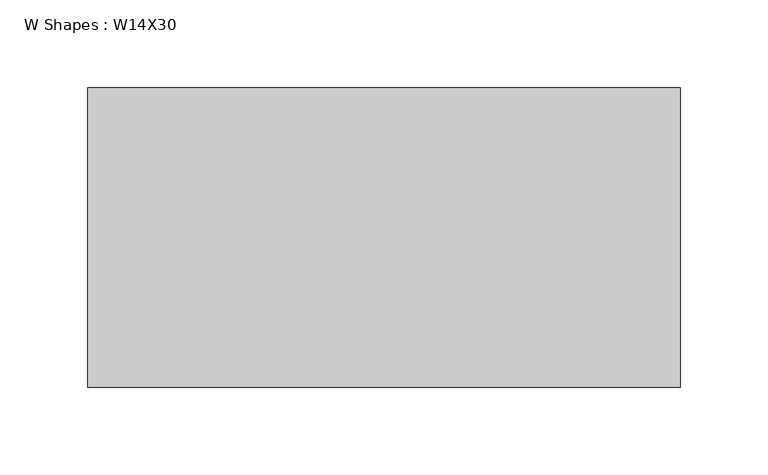
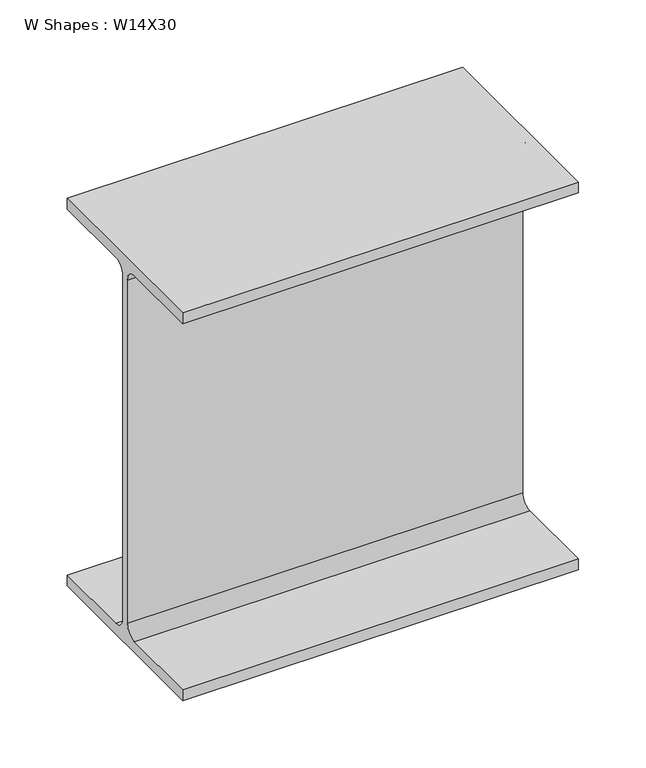
"""IFC4 building model written with IfcOpenShell, lengths in millimetres: beam geometry, W Shapes : W14X30."""

from ifc_helpers import new_model, si_unit, point, frame, frame_2d, origin, place, context, project, spatial, polyline, circle_curve, trimmed, segment, composite_curve, outline, extrude, source, transform, mapped, element, save


def w_shapes_w14x30_809da129(model_context):
    return source(origin(), model_context, "Body", "SweptSolid", [
        extrude(outline(composite_curve([segment(polyline([(85.471, -165.481), (85.471, -175.26), (-85.471, -175.26), (-85.471, -165.481), (-13.589, -165.481)]), True, "CONTINUOUS"), segment(trimmed(circle_curve(frame_2d((-13.589, -155.321)), 10.16), [point((-13.589, -165.481))], [point((-3.429, -155.321))], True, "CARTESIAN"), True, "CONTINUOUS"), segment(polyline([(-3.429, -155.321), (-3.429, 155.321)]), True, "CONTINUOUS"), segment(trimmed(circle_curve(frame_2d((-13.589, 155.321)), 10.16), [point((-3.429, 155.321))], [point((-13.589, 165.481))], True, "CARTESIAN"), True, "CONTINUOUS"), segment(polyline([(-13.589, 165.481), (-85.471, 165.481), (-85.471, 175.26), (85.471, 175.26), (85.471, 165.481), (13.589, 165.481)]), True, "CONTINUOUS"), segment(trimmed(circle_curve(frame_2d((13.589, 155.321)), 10.16), [point((13.589, 165.481))], [point((3.429, 155.321))], True, "CARTESIAN"), True, "CONTINUOUS"), segment(polyline([(3.429, 155.321), (3.429, -155.321)]), True, "CONTINUOUS"), segment(trimmed(circle_curve(frame_2d((13.589, -155.321)), 10.16), [point((3.429, -155.321))], [point((13.589, -165.481))], True, "CARTESIAN"), True, "CONTINUOUS"), segment(polyline([(13.589, -165.481), (85.471, -165.481)]), True, "CONTINUOUS")], self_intersect=False)), frame((-193.04, 0.0, 0.0), z_axis=(1.0, 0.0, 0.0), x_axis=(0.0, 1.0, 0.0)), (0.0, 0.0, 1.0), 338.2095299),
    ])


if __name__ == "__main__":
    model = new_model("IFC4")
    model_context = context("Model", 3, world=origin())
    ifc_project = project(units=[si_unit("LENGTHUNIT", "METRE", prefix="MILLI")], contexts=[model_context])
    site = spatial("IfcSite", under=ifc_project)
    building = spatial("IfcBuilding", under=site)
    placement = place(None, origin())
    w_shapes_w14x30_shape = w_shapes_w14x30_809da129(model_context)
    element("IfcBeam", 1, ObjectType="W Shapes : W14X30", at=placement, inside=building, context=model_context, shape_type="MappedRepresentation", body=[
        mapped(w_shapes_w14x30_shape, transform((0.0, 0.0, 0.0), x_axis=(1.0, 0.0, 0.0), y_axis=(0.0, 1.0, 0.0), z_axis=(0.0, 0.0, 1.0))),
    ])
    save(model, "model.ifc")

# Revit data of these elements
# Type "W Shapes : W14X30"
#   Section Name Key = "W14X30"
#   Width = 6.730"
#   Web Thickness = 0.270"
#   Web Fillet = 0.400"
#   Warping Constant = 887.00 in⁶
#   Torsional Moment of Inertia = 0.38 in⁴
#   Section Area = 8.85 in²
#   Plastic Modulus weak axis = 8.99 in³
#   Plastic Modulus strong axis = 47.30 in³
#   Perimeter = 4.441 ft²/ft
#   Nominal Weight = 30.00 lbf/ft
#   Moment of Inertia weak axis = 19.60 in⁴
#   Moment of Inertia strong axis = 291.00 in⁴
#   Height = 13.800"
#   Flange Thickness = 0.385"
#   Elastic Modulus weak axis = 5.82 in³
#   Elastic Modulus strong axis = 42.00 in³
#   Clear Web Height = 0' - 11 5/8"
#   Centroid Vertical = 6.900"
#   Centroid Horizontal = 3.365"
#   Bolt Spacing = 0' - 3 1/2"
#   Length [instance default] = 1524 mm
#   Structural Material [instance default] = Steel ASTM A992
#   Principal Axes Angle = 0
# Element 1 (IfcBeam, "W Shapes : W14X30")
#   Length = 762 mm
#   Materials on its faces: "Steel ASTM A992"
# Materials
#   "Steel ASTM A992": class "Metal", colour RGB 199 199 199, transparency 0, Description = "Structural steel 50ksi", Cost = 0
